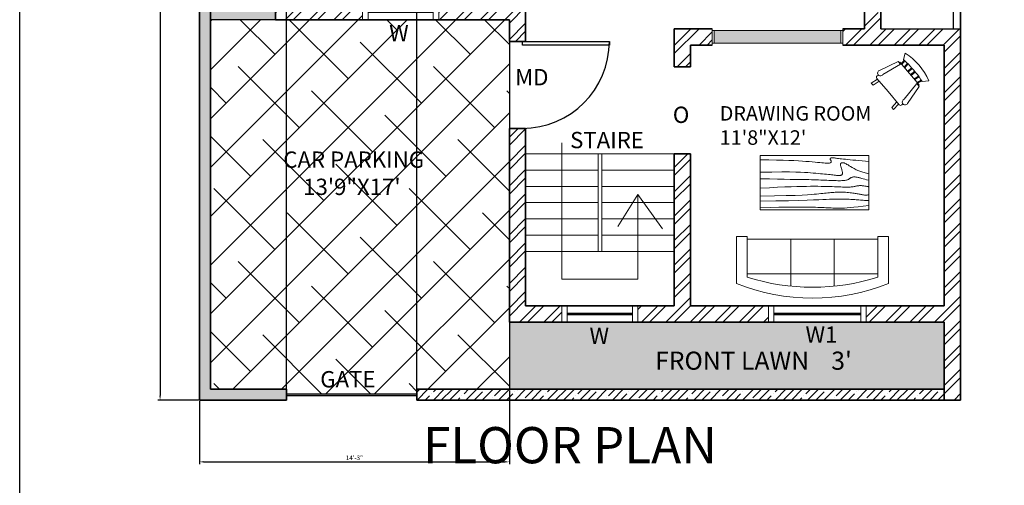
# Model space of a CAD drawing. Units: inches. Extents: x 2163 to 7246, y 928 to 2098.
# Tile 3 of 15: x 2163 to 2706, y 1365 to 1622. Entities that reach past the tile are written whole.
import ezdxf

# ---------------------------------------------------------------- set-up
doc = ezdxf.new("R2010")
doc.units = ezdxf.units.IN
for name, color, linetype, lineweight in [('A-ANNO-DIMS', 4, 'Continuous', 18), ('A-ANNO-TEXT', 7, 'Continuous', 18), ('A-ANNO-TITL', 4, 'Continuous', 30), ('A-ANNO-TTLB', 7, 'Continuous', 30), ('A-AREA-IDEN', 7, 'Continuous', 18), ('A-DOOR', 4, 'Continuous', 25), ('A-DOOR-PATT', 35, 'Continuous', 9), ('A-FLOR', 7, 'Continuous', 25), ('A-FLOR-PATT', 254, 'Continuous', 13), ('A-FLOR-STRS', 7, 'Continuous', 20), ('A-FURN', 8, 'Continuous', 18), ('A-GLAZ', 30, 'Continuous', 20), ('A-WALL', 7, 'Continuous', 35), ('A-WALL-PATT', 8, 'Continuous', 13), ('C-PROP', 7, 'Continuous', 35), ('C-PROP-PATT', 4, 'Continuous', 13)]:
    doc.layers.add(name, color=color, linetype=linetype, lineweight=lineweight)
doc.layers.add('A-GLAZ-PATT', color=141, linetype='Continuous', lineweight=9, true_color=0xadddf7)
doc.layers.add('L-PLNT-PATT', color=85, linetype='Continuous', lineweight=13, true_color=0x58ba48)
doc.styles.get("Standard").update_dxf_attribs({"font": 'arial.ttf'})
doc.dimstyles.new('ISO-25', dxfattribs={"dimtxt": 2.5, "dimasz": 2.5, "dimexe": 1.25, "dimexo": 0.625, "dimtad": 1, "dimdec": 0, "dimlunit": 3, "dimtxsty": 'Standard', "dimcen": 2.5, "dimadec": 0, "dimazin": 0, "dimtfac": 1, "dimtdec": 0, "dimtmove": 0, "dimatfit": 3, "dimfxl": 1, "dimarcsym": 0})

# ---------------------------------------------------------------- blocks, each defined once
blk = doc.blocks.new('*U2')
for p, q in [((0, 0), (0, -6)), ((40, 0), (40, -6))]:
    blk.add_line(p, q)
blk.add_lwpolyline([(0, 0), (0, 40), (1.75, 40), (1.75, 0)], close=True)
blk.add_arc((0, 0), 40, 0, 90)
blk = doc.blocks.new('Sofa - Roundback 7 ft.')
for p, q in [((-12.00002, -32.4421), (-12.00003, -6.5971)), ((11.99997, -32.4421), (11.99998, -6.5971)), ((-36.000027, -34), (-36.000027, -11.4696)), ((-35.999844, -13.3819), (35.9998, -13.3819)), ((35.99998, -34), (35.99998, -11.4696)), ((-36.000027, -32.4421), (35.99998, -32.4421))]:
    blk.add_line(p, q)
for points in [[(-36.000027, -34), (-42.000027, -34), (-42.000027, -8)], [(41.99998, -8), (41.99998, -34), (35.99998, -34)]]:
    blk.add_lwpolyline(points)
for centre, radius, start, end in [((0, -114.25), 114.25, 68.43141, 111.5686), ((-0.00001, -127.1968), 121.1968, 72.72033, 107.2797)]:
    blk.add_arc(centre, radius, start, end)
blk = doc.blocks.new('Chair - Rocking')
for p, q in [((-8, -4.5), (-10, -1.5)), ((-7.5, -4.5), (-7, -7)), ((-6.5, -7), (-7.02225, -4.43)), ((-4.5, -7), (-4.96674, -4.19951)), ((-4, -7), (-4.40532, -4.16272)), ((-1.5, -4.05012), (-1.5, -7)), ((-1, -7), (-1, -4.05012)), ((1, -7), (1, -4.04655)), ((1.5, -4.05012), (1.5, -7)), ((4, -7), (4.40187, -4.18694)), ((4.5, -7), (4.96761, -4.19437)), ((6.5, -7), (7, -4.4057)), ((7.5, -4.5), (7, -7)), ((8, -4.5), (10, -1.5)), ((-9, -7.5), (-12, -18.49999)), ((-7, -7.5), (-9, -7.5)), ((-9, -18.49999), (-7, -7.5)), ((-8.23428, -6.99939), (-8.3093, -7.47958)), ((-8.23041, -7), (8.23915, -7)), ((7, -7.5), (9, -7.5)), ((9, -18.49999), (7, -7.5)), ((8.31071, -7.48854), (8.23449, -7.00073)), ((9, -7.5), (12, -18.49999)), ((-10.36644, -20.64523), (-10.5, -21.49999)), ((10.5, -21.49999), (10.3575, -20.58798)), ((-9, -22.49999), (-9.5, -26.49999)), ((0, -22.49999), (-9.5, -22.49999)), ((-9.5, -26.49999), (-8, -26.49999)), ((-8, -26.49999), (-7.5, -22.49999)), ((0, -22.49999), (9.5, -22.49999)), ((8, -26.49999), (7.5, -22.49999)), ((9.5, -26.49999), (8, -26.49999)), ((9, -22.49999), (9.5, -26.49999))]:
    blk.add_line(p, q)
for centre, radius, start, end in [((0, -34.08333), 34.08333, 72.93847, 107.0615), ((0, -68.25004), 64.25, 93.92211, 97.15267), ((0, -68.25004), 64.25, 82.84733, 93.92211), ((-10.5, -18.99999), 1.58114, 161.5651, 18.43495), ((-9.5, -21.49999), 1, 180, 270), ((10.5, -18.99999), 1.58114, 161.5651, 18.43495), ((9.5, -21.49999), 1, 270, 0)]:
    blk.add_arc(centre, radius, start, end)
blk = doc.blocks.new('Table - Rectangular Woodgrain 60 x 30 in.')
for p, q in [((0, 0), (0, -30)), ((60, 0), (0, 0)), ((60, -30), (60, 0)), ((0, -30), (60, -30))]:
    blk.add_line(p, q)
for points in [[(0, -2.4), (4.8155, -2.418), (9.0302, -2.4688), (12.709, -2.5477), (15.9167, -2.65), (18.7181, -2.7711), (21.1781, -2.9063), (23.3616, -3.0508), (25.3333, -3.2), (27.1477, -3.3495), (28.8172, -3.4958), (30.3437, -3.636), (31.7291, -3.7667), (32.9756, -3.8849), (34.0849, -3.9875), (35.059, -4.0714), (35.9, -4.1334), (36.6114, -4.1711), (37.2041, -4.1854), (37.6906, -4.1779), (38.0833, -4.15), (38.3948, -4.1034), (38.6375, -4.0396), (38.8239, -3.9602), (38.9666, -3.8667), (39.0764, -3.7608), (39.1573, -3.6448), (39.2116, -3.521), (39.2416, -3.3917), (39.2498, -3.2593), (39.2385, -3.1261), (39.21, -2.9944), (39.1666, -2.8667), (39.111, -2.7447), (39.0468, -2.6281), (38.978, -2.5163), (38.9083, -2.4083), (38.8418, -2.3035), (38.7823, -2.201), (38.7337, -2.1001), (38.7, -2), (38.6844, -1.9003), (38.6875, -1.8021), (38.7094, -1.707), (38.75, -1.6167), (38.8094, -1.5326), (38.8875, -1.4563), (38.9844, -1.3893), (39.1, -1.3333), (39.2351, -1.2896), (39.3937, -1.2583), (39.5804, -1.2396), (39.8, -1.2333), (40.057, -1.2396), (40.3562, -1.2583), (40.7023, -1.2896), (41.1, -1.3333), (41.5547, -1.3895), (42.0755, -1.4573), (42.6721, -1.5361), (43.3542, -1.625), (44.1316, -1.7233), (45.014, -1.8302), (46.0114, -1.9449), (47.1333, -2.0667), (48.3862, -2.1947), (49.7625, -2.3281), (51.2513, -2.4663), (52.8416, -2.6083), (54.5226, -2.7535), (56.2833, -2.9011), (58.1127, -3.0501), (60, -3.2)], [(0, -9.2), (6.5759, -9.0858), (11.9385, -9.0365), (16.2527, -9.0418), (19.6833, -9.0917), (22.3952, -9.1759), (24.5531, -9.2844), (26.322, -9.4069), (27.8666, -9.5333), (29.3241, -9.6553), (30.7203, -9.7719), (32.0532, -9.8837), (33.3208, -9.9917), (34.5213, -10.0965), (35.6526, -10.199), (36.7128, -10.2999), (37.7, -10.4), (38.6129, -10.4996), (39.4531, -10.5969), (40.223, -10.6895), (40.925, -10.775), (41.5613, -10.8512), (42.1344, -10.9156), (42.6465, -10.966), (43.1, -11), (43.4976, -11.0158), (43.8437, -11.0136), (44.143, -10.9942), (44.4, -10.9583), (44.6195, -10.9069), (44.8062, -10.8406), (44.9648, -10.7603), (45.1, -10.6667), (45.2155, -10.5598), (45.3114, -10.4365), (45.3871, -10.2929), (45.4416, -10.125), (45.4743, -9.929), (45.4844, -9.7011), (45.4709, -9.4371), (45.4333, -9.1333), (45.3716, -8.7883), (45.2896, -8.4104), (45.1919, -8.0107), (45.0833, -7.6), (44.9685, -7.1893), (44.8521, -6.7896), (44.7388, -6.4117), (44.6333, -6.0667), (44.54, -5.7628), (44.4614, -5.4979), (44.4001, -5.2675), (44.3583, -5.0667), (44.3384, -4.8909), (44.3427, -4.7354), (44.3736, -4.5956), (44.4333, -4.4667), (44.5236, -4.3453), (44.6427, -4.2333), (44.7884, -4.1339), (44.9583, -4.05), (45.1501, -3.9849), (45.3614, -3.9417), (45.59, -3.9234), (45.8333, -3.9333), (46.0915, -3.9749), (46.3734, -4.0531), (46.6906, -4.1736), (47.0542, -4.3417), (47.4756, -4.5629), (47.9661, -4.8427), (48.5372, -5.1866), (49.2, -5.6), (49.9676, -6.0844), (50.8594, -6.625), (51.8965, -7.2031), (53.1, -7.8), (54.491, -8.3969), (56.0906, -8.975), (57.9199, -9.5156), (60, -10)], [(0, -12.8), (5.1847, -12.9322), (9.6213, -13.0323), (13.3963, -13.1059), (16.5958, -13.1583), (19.3063, -13.1952), (21.614, -13.2219), (23.6054, -13.2439), (25.3666, -13.2667), (26.9728, -13.2947), (28.4531, -13.3281), (29.8256, -13.3663), (31.1083, -13.4083), (32.3191, -13.4535), (33.476, -13.501), (34.597, -13.5501), (35.7, -13.6), (36.7984, -13.6497), (37.8875, -13.6979), (38.9578, -13.743), (40, -13.7833), (41.0047, -13.8174), (41.9625, -13.8438), (42.864, -13.8607), (43.7, -13.8667), (44.4631, -13.8604), (45.1552, -13.8417), (45.7801, -13.8104), (46.3416, -13.7667), (46.8439, -13.7104), (47.2906, -13.6417), (47.6858, -13.5604), (48.0333, -13.4667), (48.3375, -13.3608), (48.6042, -13.2448), (48.8396, -13.121), (49.05, -12.9917), (49.2417, -12.8593), (49.4208, -12.7261), (49.5937, -12.5944), (49.7667, -12.4667), (49.9452, -12.3451), (50.1323, -12.2313), (50.3303, -12.1268), (50.5416, -12.0333), (50.7686, -11.9524), (51.0135, -11.8854), (51.2788, -11.8341), (51.5666, -11.8), (51.8785, -11.7843), (52.2116, -11.7865), (52.562, -11.8059), (52.926, -11.8417), (53.2998, -11.8931), (53.6795, -11.9594), (54.0614, -12.0397), (54.4416, -12.1333), (54.8223, -12.2401), (55.2293, -12.3625), (55.6942, -12.5037), (56.2489, -12.6667), (56.9251, -12.8547), (57.7545, -13.0708), (58.7689, -13.3182), (60, -13.6)], [(0, -18), (5.124, -17.7273), (9.6609, -17.5057), (13.6705, -17.3303), (17.2125, -17.1958), (20.3467, -17.0973), (23.1328, -17.0297), (25.6307, -16.9878), (27.9, -16.9667), (29.9928, -16.9617), (31.9302, -16.9703), (33.7254, -16.9907), (35.3917, -17.0208), (36.9423, -17.0588), (38.3906, -17.1026), (39.7499, -17.1503), (41.0333, -17.2), (42.2519, -17.2496), (43.4073, -17.2969), (44.4986, -17.3395), (45.525, -17.375), (46.4858, -17.4012), (47.3802, -17.4156), (48.2074, -17.416), (48.9667, -17.4), (49.6583, -17.3662), (50.2872, -17.3167), (50.8595, -17.2547), (51.3812, -17.1833), (51.8584, -17.1057), (52.2971, -17.025), (52.7034, -16.9443), (53.0833, -16.8667), (53.443, -16.7951), (53.789, -16.7313), (54.128, -16.6768), (54.4666, -16.6334), (54.8115, -16.6024), (55.1693, -16.5854), (55.5465, -16.5841), (55.95, -16.6), (56.3828, -16.6337), (56.8346, -16.6823), (57.2915, -16.7418), (57.7396, -16.8084), (58.165, -16.878), (58.5539, -16.9469), (58.8924, -17.0111), (59.1666, -17.0667), (59.3679, -17.1107), (59.5078, -17.1438), (59.6032, -17.1675), (59.6708, -17.1833), (59.7275, -17.193), (59.7901, -17.1979), (59.8753, -17.1998), (60, -17.2)], [(0, -22.4), (8.0098, -22.2501), (14.4094, -22.1011), (19.4168, -21.9535), (23.25, -21.8083), (26.1269, -21.6663), (28.2656, -21.5281), (29.884, -21.3947), (31.2, -21.2667), (32.3967, -21.1448), (33.5172, -21.0292), (34.5697, -20.9198), (35.5625, -20.8167), (36.5037, -20.7198), (37.4015, -20.6292), (38.2642, -20.5448), (39.1, -20.4667), (39.9164, -20.3951), (40.7187, -20.3313), (41.5117, -20.2768), (42.3, -20.2333), (43.0883, -20.2024), (43.8812, -20.1854), (44.6836, -20.1841), (45.5, -20.2), (46.3328, -20.234), (47.1747, -20.2844), (48.0163, -20.3488), (48.8479, -20.425), (49.66, -20.5106), (50.4429, -20.6031), (51.1872, -20.7004), (51.8833, -20.8), (52.5246, -20.8999), (53.1166, -20.9995), (53.6681, -21.0983), (54.1875, -21.1958), (54.6834, -21.2919), (55.1646, -21.3859), (55.6394, -21.4777), (56.1167, -21.5667), (56.6028, -21.6515), (57.0961, -21.7266), (57.5929, -21.7852), (58.0896, -21.8208), (58.5823, -21.8268), (59.0674, -21.7964), (59.5412, -21.723), (60, -21.6)], [(0, -25.2), (8.6355, -25.0504), (15.7026, -24.9031), (21.4049, -24.7606), (25.9458, -24.625), (29.529, -24.4988), (32.3578, -24.3844), (34.6359, -24.284), (36.5667, -24.2), (38.3213, -24.1341), (39.9417, -24.0854), (41.437, -24.0523), (42.8167, -24.0333), (44.0901, -24.0268), (45.2667, -24.0313), (46.3557, -24.0451), (47.3667, -24.0667), (48.309, -24.0947), (49.1928, -24.1287), (50.0284, -24.168), (50.826, -24.2125), (51.5959, -24.2617), (52.3483, -24.3151), (53.0935, -24.3725), (53.8417, -24.4334), (54.6009, -24.497), (55.3699, -24.561), (56.1454, -24.6226), (56.9239, -24.6792), (57.7021, -24.7279), (58.4764, -24.7662), (59.2435, -24.7911), (60, -24.8)], [(0, -28.8), (5.6867, -28.6681), (10.45, -28.5698), (14.407, -28.5012), (17.675, -28.4584), (20.3711, -28.4374), (22.6125, -28.4344), (24.5164, -28.4455), (26.2, -28.4667), (27.762, -28.4947), (29.2276, -28.5281), (30.6033, -28.5663), (31.8958, -28.6084), (33.1118, -28.6535), (34.2578, -28.7011), (35.3405, -28.7501), (36.3666, -28.8), (37.3443, -28.8497), (38.288, -28.8974), (39.2137, -28.9412), (40.1375, -28.9792), (41.0753, -29.0093), (42.0432, -29.0297), (43.0572, -29.0384), (44.1333, -29.0333), (45.2936, -29.0114), (46.5843, -28.9641), (48.0579, -28.8816), (49.7666, -28.7542), (51.7629, -28.5721), (54.0989, -28.3255), (56.8272, -28.0048), (60, -27.6)]]:
    blk.add_lwpolyline(points)
blk = doc.blocks.new('*D20')
at = {"layer": 'A-ANNO-DIMS', "color": 0, "lineweight": -2, "transparency": 16777216}
for p, q in [((2261.22, 2012.07), (2238.85, 2012.07)), ((2240.1, 2009.57), (2240.1, 1414.57)), ((2261.22, 1412.07), (2238.85, 1412.07))]:
    blk.add_line(p, q, dxfattribs=at)
at = {"layer": 'A-ANNO-DIMS', "color": 0, "transparency": 16777216}
for points in [[(2239.68, 2009.57), (2240.52, 2009.57), (2240.1, 2012.07)], [(2239.68, 1414.57), (2240.52, 1414.57), (2240.1, 1412.07)]]:
    blk.add_solid(points, dxfattribs=at)
at = {"layer": 'Defpoints', "color": 0, "transparency": 16777216}
for p in [(2261.84, 2012.07), (2240.1, 1412.07), (2261.84, 1412.07)]:
    blk.add_point(p, dxfattribs=at)
at = {"layer": 'A-ANNO-DIMS', "color": 0, "transparency": 16777216, "insert": (2231.81, 1712.07), "char_height": 2.5, "attachment_point": 5, "rotation": 90}
blk.add_mtext("{\\H6x;50'}", dxfattribs=at)
blk = doc.blocks.new('WIN-36-PLAN')
for p, q in [((0, 9), (0, 0)), ((3, 9), (3, 0)), ((39, 9), (39, 0)), ((42, 9), (42, 0)), ((3, 5), (39, 5)), ((3, 4.5), (39, 4.5)), ((3, 4), (39, 4))]:
    blk.add_line(p, q)
blk = doc.blocks.new('WIN-48-PLAN')
for p, q in [((0, 9), (0, 0)), ((3, 9), (3, 0)), ((51, 9), (51, 0)), ((54, 9), (54, 0)), ((3, 5), (51, 5)), ((3, 4.5), (51, 4.5)), ((3, 4), (51, 4))]:
    blk.add_line(p, q)
blk = doc.blocks.new('TABLE-60X30-GRAIN')
for p, q in [((0, 30), (0, 0)), ((60, 30), (0, 30)), ((60, 0), (60, 30)), ((0, 0), (60, 0))]:
    blk.add_line(p, q)
for points in [[(0, 27.6), (4.8155, 27.582), (9.0302, 27.5312), (12.709, 27.4523), (15.9167, 27.35), (18.7181, 27.2289), (21.1781, 27.0937), (23.3616, 26.9492), (25.3333, 26.8), (27.1477, 26.6505), (28.8172, 26.5042), (30.3437, 26.364), (31.7291, 26.2333), (32.9756, 26.1151), (34.0849, 26.0125), (35.059, 25.9286), (35.9, 25.8666), (36.6114, 25.8289), (37.2041, 25.8146), (37.6906, 25.8221), (38.0833, 25.85), (38.3948, 25.8966), (38.6375, 25.9604), (38.8239, 26.0398), (38.9666, 26.1333), (39.0764, 26.2392), (39.1573, 26.3552), (39.2116, 26.479), (39.2416, 26.6083), (39.2498, 26.7407), (39.2385, 26.8739), (39.21, 27.0056), (39.1666, 27.1333), (39.111, 27.2553), (39.0468, 27.3719), (38.978, 27.4837), (38.9083, 27.5917), (38.8418, 27.6965), (38.7823, 27.799), (38.7337, 27.8999), (38.7, 28), (38.6844, 28.0997), (38.6875, 28.1979), (38.7094, 28.293), (38.75, 28.3833), (38.8094, 28.4674), (38.8875, 28.5437), (38.9844, 28.6107), (39.1, 28.6667), (39.2351, 28.7104), (39.3937, 28.7417), (39.5804, 28.7604), (39.8, 28.7667), (40.057, 28.7604), (40.3562, 28.7417), (40.7023, 28.7104), (41.1, 28.6667), (41.5547, 28.6105), (42.0755, 28.5427), (42.6721, 28.4639), (43.3542, 28.375), (44.1316, 28.2767), (45.014, 28.1698), (46.0114, 28.0551), (47.1333, 27.9333), (48.3862, 27.8053), (49.7625, 27.6719), (51.2513, 27.5337), (52.8416, 27.3917), (54.5226, 27.2465), (56.2833, 27.0989), (58.1127, 26.9499), (60, 26.8)], [(0, 20.8), (6.5759, 20.9142), (11.9385, 20.9635), (16.2527, 20.9582), (19.6833, 20.9083), (22.3952, 20.8241), (24.5531, 20.7156), (26.322, 20.5931), (27.8666, 20.4667), (29.3241, 20.3447), (30.7203, 20.2281), (32.0532, 20.1163), (33.3208, 20.0083), (34.5213, 19.9035), (35.6526, 19.801), (36.7128, 19.7001), (37.7, 19.6), (38.6129, 19.5004), (39.4531, 19.4031), (40.223, 19.3105), (40.925, 19.225), (41.5613, 19.1488), (42.1344, 19.0844), (42.6465, 19.034), (43.1, 19), (43.4976, 18.9842), (43.8437, 18.9864), (44.143, 19.0058), (44.4, 19.0417), (44.6195, 19.0931), (44.8062, 19.1594), (44.9648, 19.2397), (45.1, 19.3333), (45.2155, 19.4402), (45.3114, 19.5635), (45.3871, 19.7071), (45.4416, 19.875), (45.4743, 20.071), (45.4844, 20.2989), (45.4709, 20.5629), (45.4333, 20.8667), (45.3716, 21.2117), (45.2896, 21.5896), (45.1919, 21.9893), (45.0833, 22.4), (44.9685, 22.8107), (44.8521, 23.2104), (44.7388, 23.5883), (44.6333, 23.9333), (44.54, 24.2372), (44.4614, 24.5021), (44.4001, 24.7325), (44.3583, 24.9333), (44.3384, 25.1091), (44.3427, 25.2646), (44.3736, 25.4044), (44.4333, 25.5333), (44.5236, 25.6547), (44.6427, 25.7667), (44.7884, 25.8661), (44.9583, 25.95), (45.1501, 26.0151), (45.3614, 26.0583), (45.59, 26.0766), (45.8333, 26.0667), (46.0915, 26.0251), (46.3734, 25.9469), (46.6906, 25.8264), (47.0542, 25.6583), (47.4756, 25.4371), (47.9661, 25.1573), (48.5372, 24.8134), (49.2, 24.4), (49.9676, 23.9156), (50.8594, 23.375), (51.8965, 22.7969), (53.1, 22.2), (54.491, 21.6031), (56.0906, 21.025), (57.9199, 20.4844), (60, 20)], [(0, 17.2), (5.1847, 17.0678), (9.6213, 16.9677), (13.3963, 16.8941), (16.5958, 16.8417), (19.3063, 16.8048), (21.614, 16.7781), (23.6054, 16.7561), (25.3666, 16.7333), (26.9728, 16.7053), (28.4531, 16.6719), (29.8256, 16.6337), (31.1083, 16.5917), (32.3191, 16.5465), (33.476, 16.499), (34.597, 16.4499), (35.7, 16.4), (36.7984, 16.3503), (37.8875, 16.3021), (38.9578, 16.257), (40, 16.2167), (41.0047, 16.1826), (41.9625, 16.1562), (42.864, 16.1393), (43.7, 16.1333), (44.4631, 16.1396), (45.1552, 16.1583), (45.7801, 16.1896), (46.3416, 16.2333), (46.8439, 16.2896), (47.2906, 16.3583), (47.6858, 16.4396), (48.0333, 16.5333), (48.3375, 16.6392), (48.6042, 16.7552), (48.8396, 16.879), (49.05, 17.0083), (49.2417, 17.1407), (49.4208, 17.2739), (49.5937, 17.4056), (49.7667, 17.5333), (49.9452, 17.6549), (50.1323, 17.7687), (50.3303, 17.8732), (50.5416, 17.9667), (50.7686, 18.0476), (51.0135, 18.1146), (51.2788, 18.1659), (51.5666, 18.2), (51.8785, 18.2157), (52.2116, 18.2135), (52.562, 18.1941), (52.926, 18.1583), (53.2998, 18.1069), (53.6795, 18.0406), (54.0614, 17.9603), (54.4416, 17.8667), (54.8223, 17.7599), (55.2293, 17.6375), (55.6942, 17.4963), (56.2489, 17.3333), (56.9251, 17.1453), (57.7545, 16.9292), (58.7689, 16.6818), (60, 16.4)], [(0, 12), (5.124, 12.2727), (9.6609, 12.4943), (13.6705, 12.6697), (17.2125, 12.8042), (20.3467, 12.9027), (23.1328, 12.9703), (25.6307, 13.0122), (27.9, 13.0333), (29.9928, 13.0383), (31.9302, 13.0297), (33.7254, 13.0093), (35.3917, 12.9792), (36.9423, 12.9412), (38.3906, 12.8974), (39.7499, 12.8497), (41.0333, 12.8), (42.2519, 12.7504), (43.4073, 12.7031), (44.4986, 12.6605), (45.525, 12.625), (46.4858, 12.5988), (47.3802, 12.5844), (48.2074, 12.584), (48.9667, 12.6), (49.6583, 12.6338), (50.2872, 12.6833), (50.8595, 12.7453), (51.3812, 12.8167), (51.8584, 12.8943), (52.2971, 12.975), (52.7034, 13.0557), (53.0833, 13.1333), (53.443, 13.2049), (53.789, 13.2687), (54.128, 13.3232), (54.4666, 13.3666), (54.8115, 13.3976), (55.1693, 13.4146), (55.5465, 13.4159), (55.95, 13.4), (56.3828, 13.3663), (56.8346, 13.3177), (57.2915, 13.2582), (57.7396, 13.1916), (58.165, 13.122), (58.5539, 13.0531), (58.8924, 12.9889), (59.1666, 12.9333), (59.3679, 12.8893), (59.5078, 12.8562), (59.6032, 12.8325), (59.6708, 12.8167), (59.7275, 12.807), (59.7901, 12.8021), (59.8753, 12.8002), (60, 12.8)], [(0, 7.6), (8.0098, 7.7499), (14.4094, 7.8989), (19.4168, 8.0465), (23.25, 8.1917), (26.1269, 8.3337), (28.2656, 8.4719), (29.884, 8.6053), (31.2, 8.7333), (32.3967, 8.8552), (33.5172, 8.9708), (34.5697, 9.0802), (35.5625, 9.1833), (36.5037, 9.2802), (37.4015, 9.3708), (38.2642, 9.4552), (39.1, 9.5333), (39.9164, 9.6049), (40.7187, 9.6687), (41.5117, 9.7232), (42.3, 9.7667), (43.0883, 9.7976), (43.8812, 9.8146), (44.6836, 9.8159), (45.5, 9.8), (46.3328, 9.766), (47.1747, 9.7156), (48.0163, 9.6512), (48.8479, 9.575), (49.66, 9.4894), (50.4429, 9.3969), (51.1872, 9.2996), (51.8833, 9.2), (52.5246, 9.1001), (53.1166, 9.0005), (53.6681, 8.9017), (54.1875, 8.8042), (54.6834, 8.7081), (55.1646, 8.6141), (55.6394, 8.5223), (56.1167, 8.4333), (56.6028, 8.3485), (57.0961, 8.2734), (57.5929, 8.2148), (58.0896, 8.1792), (58.5823, 8.1732), (59.0674, 8.2036), (59.5412, 8.277), (60, 8.4)], [(0, 4.8), (8.6355, 4.9496), (15.7026, 5.0969), (21.4049, 5.2394), (25.9458, 5.375), (29.529, 5.5012), (32.3578, 5.6156), (34.6359, 5.716), (36.5667, 5.8), (38.3213, 5.8659), (39.9417, 5.9146), (41.437, 5.9477), (42.8167, 5.9667), (44.0901, 5.9732), (45.2667, 5.9687), (46.3557, 5.9549), (47.3667, 5.9333), (48.309, 5.9053), (49.1928, 5.8713), (50.0284, 5.832), (50.826, 5.7875), (51.5959, 5.7383), (52.3483, 5.6849), (53.0935, 5.6275), (53.8417, 5.5666), (54.6009, 5.503), (55.3699, 5.439), (56.1454, 5.3774), (56.9239, 5.3208), (57.7021, 5.2721), (58.4764, 5.2338), (59.2435, 5.2089), (60, 5.2)], [(0, 1.2), (5.6867, 1.3319), (10.45, 1.4302), (14.407, 1.4988), (17.675, 1.5416), (20.3711, 1.5626), (22.6125, 1.5656), (24.5164, 1.5545), (26.2, 1.5333), (27.762, 1.5053), (29.2276, 1.4719), (30.6033, 1.4337), (31.8958, 1.3916), (33.1118, 1.3465), (34.2578, 1.2989), (35.3405, 1.2499), (36.3666, 1.2), (37.3443, 1.1503), (38.288, 1.1026), (39.2137, 1.0588), (40.1375, 1.0208), (41.0753, 0.9907), (42.0432, 0.9703), (43.0572, 0.9616), (44.1333, 0.9667), (45.2936, 0.9886), (46.5843, 1.0359), (48.0579, 1.1184), (49.7666, 1.2458), (51.7629, 1.4279), (54.0989, 1.6745), (56.8272, 1.9952), (60, 2.4)]]:
    blk.add_lwpolyline(points)
blk = doc.blocks.new('*D77')
at = {"layer": 'A-ANNO-DIMS', "color": 0, "lineweight": -2, "transparency": 16777216}
for p, q in [((2432.84, 1417.45), (2432.84, 1376.72)), ((2261.84, 1411.45), (2261.84, 1376.72)), ((2264.34, 1377.97), (2430.34, 1377.97))]:
    blk.add_line(p, q, dxfattribs=at)
at = {"layer": 'A-ANNO-DIMS', "color": 0, "transparency": 16777216}
for points in [[(2264.34, 1378.39), (2264.34, 1377.56), (2261.84, 1377.97)], [(2430.34, 1378.39), (2430.34, 1377.56), (2432.84, 1377.97)]]:
    blk.add_solid(points, dxfattribs=at)
at = {"layer": 'Defpoints', "color": 0, "transparency": 16777216}
for p in [(2432.84, 1418.07), (2261.84, 1412.07), (2432.84, 1377.97)]:
    blk.add_point(p, dxfattribs=at)
at = {"layer": 'A-ANNO-DIMS', "color": 0, "transparency": 16777216, "insert": (2347.34, 1379.88), "char_height": 2.5, "attachment_point": 5}
blk.add_mtext('14\'-3"', dxfattribs=at)
blk = doc.blocks.new('*D78')
at = {"layer": 'A-ANNO-DIMS', "color": 0, "lineweight": -2, "transparency": 16777216}
for p, q in [((2309.84, 1412.7), (2309.84, 2047.42)), ((2312.34, 2046.17), (2379.34, 2046.17)), ((2381.84, 1412.7), (2381.84, 2047.42))]:
    blk.add_line(p, q, dxfattribs=at)
at = {"layer": 'A-ANNO-DIMS', "color": 0, "transparency": 16777216}
for points in [[(2312.34, 2046.59), (2312.34, 2045.76), (2309.84, 2046.17)], [(2379.34, 2046.59), (2379.34, 2045.76), (2381.84, 2046.17)]]:
    blk.add_solid(points, dxfattribs=at)
at = {"layer": 'Defpoints', "color": 0, "transparency": 16777216}
for p in [(2381.84, 2046.17), (2309.84, 1412.07), (2381.84, 1412.07)]:
    blk.add_point(p, dxfattribs=at)
at = {"layer": 'A-ANNO-DIMS', "color": 0, "transparency": 16777216, "insert": (2345.84, 2048.07), "char_height": 2.5, "attachment_point": 5}
blk.add_mtext('6\'-0"', dxfattribs=at)

msp = doc.modelspace()

# ---------------------------------------------------------------- hatches: boundary and pattern name
at = {"layer": 'A-DOOR-PATT'}
h = msp.add_hatch(color=256, dxfattribs=at)
h.dxf.hatch_style = 1
h.paths.add_polyline_path([(2381.84, 1415.57), (2309.84, 1415.57), (2309.84, 1414.57), (2381.84, 1414.57)])
at = {"layer": 'A-FLOR-PATT'}
h = msp.add_hatch(dxfattribs=at)
h.set_pattern_fill('ANSI38', color=256, scale=6)
h.paths.add_polyline_path([(2381.84, 1415.57), (2381.84, 1418.07), (2432.84, 1418.07), (2432.84, 1455.07), (2432.84, 1562.07), (2432.84, 1610.07), (2432.84, 1622.07), (2303.84, 1622.07), (2267.84, 1622.07), (2267.84, 1418.07), (2309.84, 1418.07), (2309.84, 1415.57)])
h.paths.add_polyline_path([(2325.55, 1414.01), (2364.28, 1414.01), (2364.28, 1432.56), (2325.55, 1432.56)], flags=9)
h.paths.add_polyline_path([(2305.2, 1520.21), (2396.33, 1520.21), (2396.33, 1553.79), (2305.2, 1553.79)], flags=24)
at = {"layer": 'A-GLAZ-PATT'}
h = msp.add_hatch(color=256, dxfattribs=at)
h.dxf.hatch_style = 1
h.paths.add_polyline_path([(2615.84, 1616.07), (2545.84, 1616.07), (2545.84, 1609.07), (2615.84, 1609.07)])
at = {"layer": 'A-WALL-PATT'}
h = msp.add_hatch(dxfattribs=at)
h.set_pattern_fill('ANSI32', color=256)
h.paths.add_polyline_path([(2461.84, 1464.07), (2441.84, 1464.07), (2441.84, 1562.07), (2432.84, 1562.07), (2432.84, 1455.07), (2461.84, 1455.07)])
h.paths.add_polyline_path([(2575.84, 1464.07), (2532.84, 1464.07), (2532.84, 1548.07), (2523.84, 1548.07), (2523.84, 1464.07), (2503.84, 1464.07), (2503.84, 1455.07), (2575.84, 1455.07)])
h.paths.add_polyline_path([(2681.84, 1617.07), (2637.84, 1617.07), (2637.84, 1626.07), (2628.84, 1626.07), (2628.84, 1617.07), (2616.84, 1617.07), (2616.84, 1608.07), (2672.84, 1608.07), (2672.84, 1464.07), (2629.84, 1464.07), (2629.84, 1455.07), (2672.84, 1455.07), (2672.84, 1412.07), (2681.84, 1412.07)])
h.paths.add_polyline_path([(2544.84, 1617.07), (2523.84, 1617.07), (2523.84, 1596.07), (2532.84, 1596.07), (2532.84, 1608.07), (2544.84, 1608.07)])
h.paths.add_polyline_path([(2441.84, 1682.07), (2432.84, 1682.07), (2432.84, 1631.07), (2393.84, 1631.07), (2393.84, 1622.07), (2432.84, 1622.07), (2432.84, 1610.07), (2441.84, 1610.07)])
h.paths.add_polyline_path([(2441.84, 1736.07), (2424.84, 1736.07), (2424.84, 1808.07), (2436.84, 1808.07), (2436.84, 1817.07), (2406.84, 1817.07), (2406.84, 1808.07), (2415.84, 1808.07), (2415.84, 1736.07), (2331.84, 1736.07), (2331.84, 1757.07), (2322.84, 1757.07), (2322.84, 1736.07), (2303.84, 1736.07), (2303.84, 1700.07), (2312.84, 1700.07), (2312.84, 1727.07), (2432.84, 1727.07), (2432.84, 1718.07), (2441.84, 1718.07)])
h.paths.add_polyline_path([(2351.84, 1631.07), (2312.84, 1631.07), (2312.84, 1658.07), (2303.84, 1658.07), (2303.84, 1622.07), (2351.84, 1622.07)])
at = {"layer": 'C-PROP-PATT'}
h = msp.add_hatch(dxfattribs=at)
h.set_pattern_fill('ANSI35', color=256)
h.paths.add_polyline_path([(2309.84, 1418.07), (2267.84, 1418.07), (2267.84, 2006.07), (2579.84, 2006.07), (2579.84, 2012.07), (2261.84, 2012.07), (2261.84, 1412.07), (2309.84, 1412.07)])
h = msp.add_hatch(dxfattribs=at)
h.set_pattern_fill('ANSI35', color=256)
h.paths.add_polyline_path([(2672.84, 1418.07), (2381.84, 1418.07), (2381.84, 1412.07), (2672.84, 1412.07)])
at = {"layer": 'L-PLNT-PATT'}
h = msp.add_hatch(dxfattribs=at)
h.set_pattern_fill('CROSS', color=256)
h.paths.add_polyline_path([(2579.84, 2006.07), (2267.84, 2006.07), (2267.84, 1622.07), (2303.84, 1622.07), (2303.84, 1736.07), (2322.84, 1736.07), (2322.84, 1808.07), (2303.84, 1808.07), (2303.84, 1970.07), (2579.84, 1970.07)])
h.paths.add_polyline_path([(2672.84, 1455.07), (2432.84, 1455.07), (2432.84, 1418.07), (2672.84, 1418.07)])
h.paths.add_polyline_path([(2291.95, 1715.76), (2291.95, 1812.79), (2273.41, 1812.79), (2273.41, 1715.76)], flags=24)
h.paths.add_polyline_path([(2413.78, 1978.86), (2515.7, 1978.86), (2515.7, 1997.41), (2413.78, 1997.41)], flags=24)
h.paths.add_polyline_path([(2509.67, 1423.19), (2632.98, 1423.19), (2632.98, 1443.8), (2509.67, 1443.8)], flags=24)

# ---------------------------------------------------------------- linework, layer by layer
at = {"layer": 'A-ANNO-TTLB'}
msp.add_lwpolyline([(2162.62, 2098.21), (3633.38, 2098.21), (3633.38, 928.48), (2162.62, 928.48)], close=True, dxfattribs=at)
at = {"layer": 'A-DOOR'}
for p, q in [((2432.84, 1610.07), (2432.84, 1562.07)), ((2309.84, 1415.57), (2381.84, 1415.57)), ((2309.84, 1414.57), (2381.84, 1414.57))]:
    msp.add_line(p, q, dxfattribs=at)
at = {"layer": 'A-FLOR'}
for p, q in [((2677.84, 1761.07), (2677.84, 1617.07)), ((2303.84, 1622.07), (2267.84, 1622.07)), ((2637.84, 1617.07), (2681.84, 1617.07)), ((2432.84, 1455.07), (2432.84, 1418.07))]:
    msp.add_line(p, q, dxfattribs=at)
at = {"layer": 'A-FLOR-STRS'}
for p, q in [((2461.84, 1554.09), (2461.84, 1478.74)), ((2523.84, 1548.07), (2441.84, 1548.07)), ((2481.84, 1494.07), (2481.84, 1548.07)), ((2483.84, 1494.07), (2483.84, 1548.07)), ((2441.84, 1539.07), (2481.84, 1539.07)), ((2483.84, 1539.07), (2523.84, 1539.07)), ((2441.84, 1530.07), (2481.84, 1530.07)), ((2483.84, 1530.07), (2523.84, 1530.07)), ((2503.84, 1525.63), (2492.67, 1507.88)), ((2503.84, 1478.74), (2503.84, 1525.63)), ((2503.84, 1525.63), (2517.38, 1506.65)), ((2441.84, 1521.07), (2481.84, 1521.07)), ((2483.84, 1521.07), (2523.84, 1521.07)), ((2441.84, 1512.07), (2481.84, 1512.07)), ((2483.84, 1512.07), (2523.84, 1512.07)), ((2441.84, 1503.07), (2481.84, 1503.07)), ((2483.84, 1503.07), (2523.84, 1503.07)), ((2441.84, 1494.07), (2523.84, 1494.07)), ((2461.84, 1478.74), (2503.84, 1478.74))]:
    msp.add_line(p, q, dxfattribs=at)
at = {"layer": 'A-GLAZ'}
for p, q in [((2544.84, 1617.07), (2544.84, 1608.07)), ((2544.84, 1616.07), (2616.84, 1616.07)), ((2545.84, 1616.07), (2545.84, 1609.07)), ((2615.84, 1609.07), (2615.84, 1616.07)), ((2616.84, 1608.07), (2616.84, 1617.07)), ((2544.84, 1609.07), (2616.84, 1609.07))]:
    msp.add_line(p, q, dxfattribs=at)
at = {"layer": 'A-WALL'}
for p, q in [((2628.84, 1617.07), (2628.84, 1761.07)), ((2637.84, 1617.07), (2637.84, 1761.07)), ((2303.84, 1622.07), (2303.84, 1736.07)), ((2441.84, 1610.07), (2441.84, 1682.07)), ((2303.84, 1622.07), (2432.84, 1622.07)), ((2432.84, 1610.07), (2432.84, 1622.07)), ((2523.84, 1617.07), (2523.84, 1596.07)), ((2523.84, 1617.07), (2544.84, 1617.07)), ((2616.84, 1617.07), (2628.84, 1617.07)), ((2432.84, 1610.07), (2441.84, 1610.07)), ((2532.84, 1608.07), (2532.84, 1596.07)), ((2532.84, 1608.07), (2544.84, 1608.07)), ((2616.84, 1608.07), (2672.84, 1608.07)), ((2672.84, 1608.07), (2672.84, 1464.07)), ((2523.84, 1596.07), (2532.84, 1596.07)), ((2432.84, 1455.07), (2432.84, 1562.07)), ((2432.84, 1562.07), (2441.84, 1562.07)), ((2441.84, 1464.07), (2441.84, 1562.07)), ((2523.84, 1548.07), (2523.84, 1464.07)), ((2523.84, 1548.07), (2532.84, 1548.07)), ((2532.84, 1548.07), (2532.84, 1464.07)), ((2441.84, 1464.07), (2523.84, 1464.07)), ((2532.84, 1464.07), (2672.84, 1464.07)), ((2432.84, 1455.07), (2672.84, 1455.07))]:
    msp.add_line(p, q, dxfattribs=at)
at = {"layer": 'C-PROP'}
for p, q in [((2261.84, 1412.07), (2261.84, 2012.07)), ((2681.84, 2012.07), (2681.84, 1412.07)), ((2267.84, 1418.07), (2267.84, 2006.07)), ((2672.84, 1455.07), (2672.84, 1412.07)), ((2309.84, 1418.07), (2267.84, 1418.07)), ((2309.84, 1412.07), (2309.84, 1418.07)), ((2672.84, 1418.07), (2381.84, 1418.07)), ((2381.84, 1412.07), (2381.84, 1418.07)), ((2672.84, 1418.07), (2532.84, 1418.07)), ((2309.84, 1412.07), (2261.84, 1412.07)), ((2681.84, 1412.07), (2381.84, 1412.07))]:
    msp.add_line(p, q, dxfattribs=at)

# ---------------------------------------------------------------- block references
at = {"layer": 'A-DOOR', "xscale": 1.199999999999999, "yscale": 1.199999999999999, "zscale": 1.199999999999999, "rotation": 270}
msp.add_blockref('*U2', (2440.04, 1610.07), dxfattribs=at)
at = {"layer": 'A-FURN'}
for name, p, rotation in [('Chair - Rocking', (2658.94, 1596.96), 310.4239173852844), ('Sofa - Roundback 7 ft.', (2600.16, 1468.39), 180)]:
    msp.add_blockref(name, p, dxfattribs=dict(at, rotation=rotation))
for name, p in [('Table - Rectangular Woodgrain 60 x 30 in.', (2571.2, 1547.06)), ('TABLE-60X30-GRAIN', (2571.2, 1517.06)), ('TABLE-60X30-GRAIN', (2571.2, 1517.06)), ('TABLE-60X30-GRAIN', (2571.2, 1517.06)), ('TABLE-60X30-GRAIN', (2571.2, 1517.06)), ('TABLE-60X30-GRAIN', (2571.2, 1517.06))]:
    msp.add_blockref(name, p, dxfattribs=at)
at = {"layer": 'A-GLAZ'}
for name, p in [('WIN-36-PLAN', (2351.84, 1622.07)), ('WIN-36-PLAN', (2461.84, 1455.07)), ('WIN-48-PLAN', (2575.84, 1455.07))]:
    msp.add_blockref(name, p, dxfattribs=at)

# ---------------------------------------------------------------- texts
at = {"layer": 'A-ANNO-TEXT', "char_height": 9, "attachment_point": 1}
for s, width, insert in [('W', 361.5259, (2366.51, 1619.18)), ('MD', 361.5259, (2436.03, 1594.83)), ('O', 361.5259, (2523.06, 1574.07)), ('W', 361.5259, (2477.08, 1452.09)), ('W1', 361.5259, (2596.3, 1452.73)), ('GATE', 128.9736, (2328.47, 1428.08))]:
    msp.add_mtext_dynamic_manual_height_columns(s, width=width, gutter_width=12.5, heights=[0], dxfattribs=dict(at, insert=insert))
at = {"layer": 'A-ANNO-TITL', "insert": (2385.2, 1397.18), "char_height": 20, "attachment_point": 1}
msp.add_mtext_dynamic_manual_height_columns('FLOOR PLAN', width=571.2399, gutter_width=12.5, heights=[0], dxfattribs=at)
at = {"layer": 'A-AREA-IDEN', "attachment_point": 1}
for s, width, insert, char_height in [('DRAWING ROOM\\P11\'8"X12\'', 322.0134, (2548.96, 1574.35), 8), ('STAIRE', 128.9736, (2466.37, 1560.13), 9), ('CAR PARKING\\P    13\'9"X17\'', 530.9337, (2308.07, 1549.31), 9), ("FRONT LAWN    3'", 200.589, (2513.31, 1438.83), 10)]:
    msp.add_mtext_dynamic_manual_height_columns(s, width=width, gutter_width=12.5, heights=[0], dxfattribs=dict(at, insert=insert, char_height=char_height))

# ---------------------------------------------------------------- dimensions: what is measured, and where the dimension line sits
at = {"layer": 'A-ANNO-DIMS'}
for base, p1, p2, picture, middle in [((2381.84, 2046.17), (2309.84, 1412.07), (2381.84, 1412.07), '*D78', (2345.84, 2048.07)), ((2432.84, 1377.97), (2261.84, 1412.07), (2432.84, 1418.07), '*D77', (2347.34, 1379.88))]:
    dim = msp.add_linear_dim(base=base, p1=p1, p2=p2, dimstyle='ISO-25', override={"dimdec": 1, "dimlfac": 1, "dimrnd": 0, "dimzin": 1, "dimdsep": 46, "dimlunit": 4, "dimfrac": 2}, dxfattribs=at)
    dim.commit()
    dim.dimension.update_dxf_attribs({"geometry": picture, "text_midpoint": middle})
dim = msp.add_linear_dim(base=(2240.1, 1412.07), p1=(2261.84, 2012.07), p2=(2261.84, 1412.07), angle=90, text='{\\H6x;<>}', dimstyle='ISO-25', override={"dimclrd": 0, "dimclre": 0, "dimclrt": 0}, dxfattribs=at)
dim.commit()
dim.dimension.update_dxf_attribs({"geometry": '*D20', "text_midpoint": (2231.81, 1712.07)})

doc.saveas('drawing.dxf')
